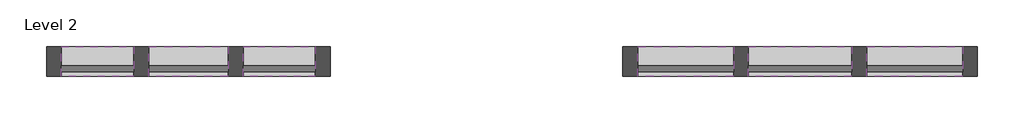
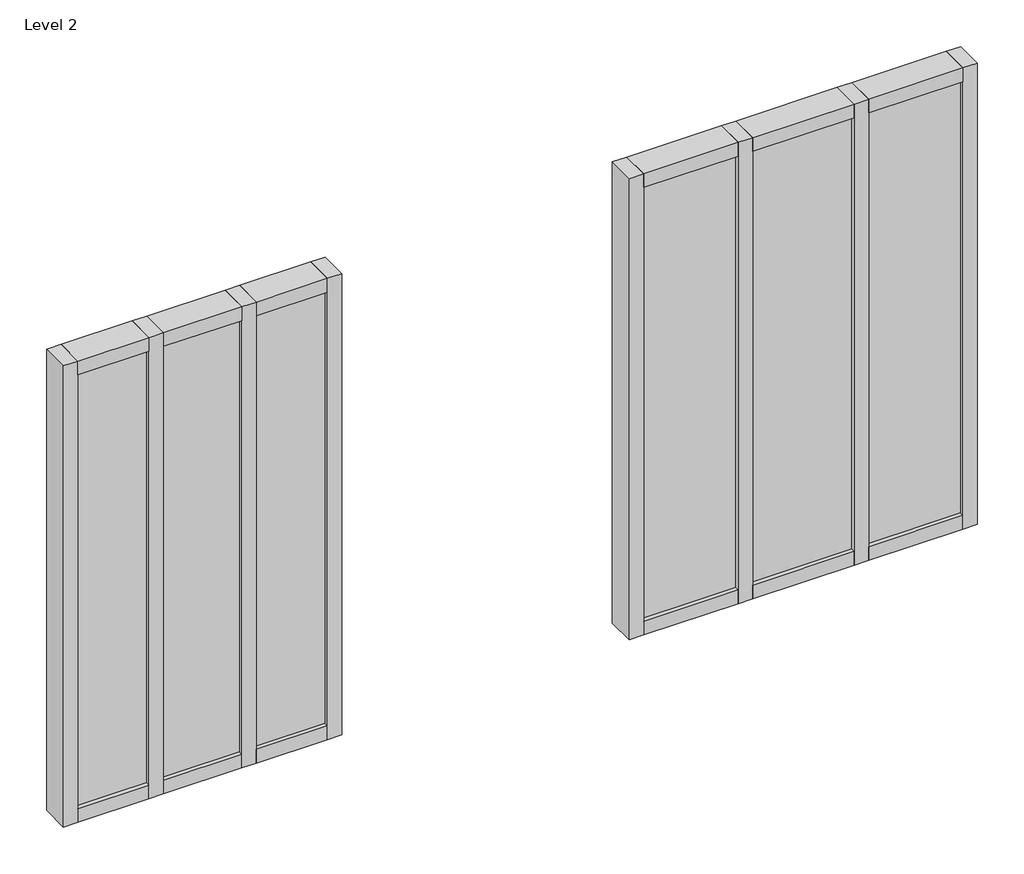
# One storey: 20 members, 6 plates.
"""IFC4 building model written with IfcOpenShell, lengths in millimetres."""

from ifc_helpers import new_model, si_unit, origin, place, context, project, spatial, transform, mapped, element, save
from components import member_dc106669, member_bc7dbe04, member_7cbddb58, member_3374d9b6, member_5ad95953, member_ff1b7d8f, system_panel_glazed_74c9e8f4, system_panel_glazed_660eca69, system_panel_glazed_45f6ab2d, system_panel_glazed_d43c1d57

model = new_model("IFC4")

# Units and contexts
model_context = context("Model", 3, world=origin())
ifc_project = project(units=[si_unit("LENGTHUNIT", "METRE", prefix="MILLI")], contexts=[model_context])

# Site, building, storey
site = spatial("IfcSite", under=ifc_project)
building = spatial("IfcBuilding", under=site)
storey = spatial("IfcBuildingStorey", under=building, Name="Level 2", Elevation=609.6)

# Members
placement = place(None, origin())
member_shape = member_dc106669(model_context)
element("IfcMember", 1, ObjectType="Rectangular Mullion : 2.5\" x 5\" rectangular", at=placement, inside=storey, context=model_context, shape_type="MappedRepresentation", body=[
    mapped(member_shape, transform((-8008.9218714, -2282.1569638, 2743.2), x_axis=(0.0, 0.0, 1.0), y_axis=(0.0, 1.0, 0.0), z_axis=(-1.0, 0.0, 0.0))),
])
element("IfcMember", 2, ObjectType="Rectangular Mullion : 2.5\" x 5\" rectangular", at=placement, inside=storey, context=model_context, shape_type="MappedRepresentation", body=[
    mapped(member_shape, transform((-7024.6718714, -2282.1569638, 2743.2), x_axis=(0.0, 0.0, 1.0), y_axis=(0.0, 1.0, 0.0), z_axis=(-1.0, 0.0, 0.0))),
])
element("IfcMember", 3, ObjectType="Rectangular Mullion : 2.5\" x 5\" rectangular", at=placement, inside=storey, context=model_context, shape_type="MappedRepresentation", body=[
    mapped(member_shape, transform((-6611.9218714, -2282.1569638, 609.6), x_axis=(0.0, 0.0, -1.0), y_axis=(0.0, 1.0, 0.0), z_axis=(1.0, 0.0, 0.0))),
])
element("IfcMember", 4, ObjectType="Rectangular Mullion : 2.5\" x 5\" rectangular", at=placement, inside=storey, context=model_context, shape_type="MappedRepresentation", body=[
    mapped(member_shape, transform((-7596.1718714, -2282.1569638, 609.6), x_axis=(0.0, 0.0, -1.0), y_axis=(0.0, 1.0, 0.0), z_axis=(1.0, 0.0, 0.0))),
])
member_2_shape = member_bc7dbe04(model_context)
element("IfcMember", 5, ObjectType="Rectangular Mullion : 2.5\" x 5\" rectangular", at=placement, inside=storey, context=model_context, shape_type="MappedRepresentation", body=[
    mapped(member_2_shape, transform((-7088.1718714, -2282.1569638, 609.6), x_axis=(0.0, 0.0, -1.0), y_axis=(0.0, 1.0, 0.0), z_axis=(1.0, 0.0, 0.0))),
])
element("IfcMember", 6, ObjectType="Rectangular Mullion : 2.5\" x 5\" rectangular", at=placement, inside=storey, context=model_context, shape_type="MappedRepresentation", body=[
    mapped(member_2_shape, transform((-7532.6718714, -2282.1569638, 2743.2), x_axis=(0.0, 0.0, 1.0), y_axis=(0.0, 1.0, 0.0), z_axis=(-1.0, 0.0, 0.0))),
])
member_3_shape = member_7cbddb58(model_context)
element("IfcMember", 7, ObjectType="Rectangular Mullion : 2.5\" x 5\" rectangular", at=placement, inside=storey, context=model_context, shape_type="MappedRepresentation", body=[
    mapped(member_3_shape, transform((-7564.4218714, -2282.1569638, 609.6), x_axis=(-1.0, 0.0, 0.0), y_axis=(0.0, 1.0, 0.0), z_axis=(0.0, 0.0, -1.0))),
])
element("IfcMember", 8, ObjectType="Rectangular Mullion : 2.5\" x 5\" rectangular", at=placement, inside=storey, context=model_context, shape_type="MappedRepresentation", body=[
    mapped(member_3_shape, transform((-7056.4218714, -2282.1569638, 609.6), x_axis=(-1.0, 0.0, 0.0), y_axis=(0.0, 1.0, 0.0), z_axis=(0.0, 0.0, -1.0))),
])
element("IfcMember", 9, ObjectType="Rectangular Mullion : 2.5\" x 5\" rectangular", at=placement, inside=storey, context=model_context, shape_type="MappedRepresentation", body=[
    mapped(member_3_shape, transform((-10142.5218714, -2282.1569638, 609.6), x_axis=(-1.0, 0.0, 0.0), y_axis=(0.0, 1.0, 0.0), z_axis=(0.0, 0.0, -1.0))),
])
element("IfcMember", 10, ObjectType="Rectangular Mullion : 2.5\" x 5\" rectangular", at=placement, inside=storey, context=model_context, shape_type="MappedRepresentation", body=[
    mapped(member_3_shape, transform((-9736.1218714, -2282.1569638, 609.6), x_axis=(-1.0, 0.0, 0.0), y_axis=(0.0, 1.0, 0.0), z_axis=(0.0, 0.0, -1.0))),
])
member_4_shape = member_3374d9b6(model_context)
element("IfcMember", 11, ObjectType="Rectangular Mullion : 2.5\" x 5\" rectangular", at=placement, inside=storey, context=model_context, shape_type="MappedRepresentation", body=[
    mapped(member_4_shape, transform((-6548.4218714, -2282.1569638, 2743.2), x_axis=(1.0, 0.0, 0.0), y_axis=(0.0, 1.0, 0.0), z_axis=(0.0, 0.0, 1.0))),
])
element("IfcMember", 12, ObjectType="Rectangular Mullion : 2.5\" x 5\" rectangular", at=placement, inside=storey, context=model_context, shape_type="MappedRepresentation", body=[
    mapped(member_4_shape, transform((-9329.7218714, -2282.1569638, 2743.2), x_axis=(1.0, 0.0, 0.0), y_axis=(0.0, 1.0, 0.0), z_axis=(0.0, 0.0, 1.0))),
])
element("IfcMember", 13, ObjectType="Rectangular Mullion : 2.5\" x 5\" rectangular", at=placement, inside=storey, context=model_context, shape_type="MappedRepresentation", body=[
    mapped(member_4_shape, transform((-8072.4218714, -2282.1569638, 609.6), x_axis=(-1.0, 0.0, 0.0), y_axis=(0.0, 1.0, 0.0), z_axis=(0.0, 0.0, -1.0))),
])
element("IfcMember", 14, ObjectType="Rectangular Mullion : 2.5\" x 5\" rectangular", at=placement, inside=storey, context=model_context, shape_type="MappedRepresentation", body=[
    mapped(member_4_shape, transform((-10548.9218714, -2282.1569638, 609.6), x_axis=(-1.0, 0.0, 0.0), y_axis=(0.0, 1.0, 0.0), z_axis=(0.0, 0.0, -1.0))),
])
member_5_shape = member_5ad95953(model_context)
element("IfcMember", 15, ObjectType="Rectangular Mullion : 2.5\" x 5\" rectangular", at=placement, inside=storey, context=model_context, shape_type="MappedRepresentation", body=[
    mapped(member_5_shape, transform((-10485.4218714, -2282.1569638, 2743.2), x_axis=(0.0, 0.0, 1.0), y_axis=(0.0, 1.0, 0.0), z_axis=(-1.0, 0.0, 0.0))),
])
element("IfcMember", 16, ObjectType="Rectangular Mullion : 2.5\" x 5\" rectangular", at=placement, inside=storey, context=model_context, shape_type="MappedRepresentation", body=[
    mapped(member_5_shape, transform((-9704.3718714, -2282.1569638, 2743.2), x_axis=(0.0, 0.0, 1.0), y_axis=(0.0, 1.0, 0.0), z_axis=(-1.0, 0.0, 0.0))),
])
element("IfcMember", 17, ObjectType="Rectangular Mullion : 2.5\" x 5\" rectangular", at=placement, inside=storey, context=model_context, shape_type="MappedRepresentation", body=[
    mapped(member_5_shape, transform((-9393.2218714, -2282.1569638, 609.6), x_axis=(0.0, 0.0, -1.0), y_axis=(0.0, 1.0, 0.0), z_axis=(1.0, 0.0, 0.0))),
])
element("IfcMember", 18, ObjectType="Rectangular Mullion : 2.5\" x 5\" rectangular", at=placement, inside=storey, context=model_context, shape_type="MappedRepresentation", body=[
    mapped(member_5_shape, transform((-10174.2718714, -2282.1569638, 609.6), x_axis=(0.0, 0.0, -1.0), y_axis=(0.0, 1.0, 0.0), z_axis=(1.0, 0.0, 0.0))),
])
member_6_shape = member_ff1b7d8f(model_context)
element("IfcMember", 19, ObjectType="Rectangular Mullion : 2.5\" x 5\" rectangular", at=placement, inside=storey, context=model_context, shape_type="MappedRepresentation", body=[
    mapped(member_6_shape, transform((-9767.8718714, -2282.1569638, 609.6), x_axis=(0.0, 0.0, -1.0), y_axis=(0.0, 1.0, 0.0), z_axis=(1.0, 0.0, 0.0))),
])
element("IfcMember", 20, ObjectType="Rectangular Mullion : 2.5\" x 5\" rectangular", at=placement, inside=storey, context=model_context, shape_type="MappedRepresentation", body=[
    mapped(member_6_shape, transform((-10110.7718714, -2282.1569638, 2743.2), x_axis=(0.0, 0.0, 1.0), y_axis=(0.0, 1.0, 0.0), z_axis=(-1.0, 0.0, 0.0))),
])

# Plates
system_panel_glazed_shape = system_panel_glazed_74c9e8f4(model_context)
element("IfcPlate", 21, ObjectType="System Panel : Glazed", at=placement, inside=storey, context=model_context, shape_type="MappedRepresentation", body=[
    mapped(system_panel_glazed_shape, transform((-6818.2968714, -2282.1569638, 673.1), x_axis=(-1.0, 0.0, 0.0), y_axis=(0.0, -1.0, 0.0), z_axis=(0.0, 0.0, 1.0))),
])
element("IfcPlate", 22, ObjectType="System Panel : Glazed", at=placement, inside=storey, context=model_context, shape_type="MappedRepresentation", body=[
    mapped(system_panel_glazed_shape, transform((-7802.5468714, -2282.1569638, 673.1), x_axis=(-1.0, 0.0, 0.0), y_axis=(0.0, -1.0, 0.0), z_axis=(0.0, 0.0, 1.0))),
])
system_panel_glazed_2_shape = system_panel_glazed_660eca69(model_context)
element("IfcPlate", 23, ObjectType="System Panel : Glazed", at=placement, inside=storey, context=model_context, shape_type="MappedRepresentation", body=[
    mapped(system_panel_glazed_2_shape, transform((-7310.4218714, -2282.1569638, 673.1), x_axis=(-1.0, 0.0, 0.0), y_axis=(0.0, -1.0, 0.0), z_axis=(0.0, 0.0, 1.0))),
])
system_panel_glazed_3_shape = system_panel_glazed_45f6ab2d(model_context)
element("IfcPlate", 24, ObjectType="System Panel : Glazed", at=placement, inside=storey, context=model_context, shape_type="MappedRepresentation", body=[
    mapped(system_panel_glazed_3_shape, transform((-9548.7968714, -2282.1569638, 673.1), x_axis=(-1.0, 0.0, 0.0), y_axis=(0.0, -1.0, 0.0), z_axis=(0.0, 0.0, 1.0))),
])
element("IfcPlate", 25, ObjectType="System Panel : Glazed", at=placement, inside=storey, context=model_context, shape_type="MappedRepresentation", body=[
    mapped(system_panel_glazed_3_shape, transform((-10329.8468714, -2282.1569638, 673.1), x_axis=(-1.0, 0.0, 0.0), y_axis=(0.0, -1.0, 0.0), z_axis=(0.0, 0.0, 1.0))),
])
system_panel_glazed_4_shape = system_panel_glazed_d43c1d57(model_context)
element("IfcPlate", 26, ObjectType="System Panel : Glazed", at=placement, inside=storey, context=model_context, shape_type="MappedRepresentation", body=[
    mapped(system_panel_glazed_4_shape, transform((-9939.3218714, -2282.1569638, 673.1), x_axis=(-1.0, 0.0, 0.0), y_axis=(0.0, -1.0, 0.0), z_axis=(0.0, 0.0, 1.0))),
])

save(model, "model.ifc")

# Revit data of these elements
# Type "Rectangular Mullion : 2.5\" x 5\" rectangular"
#   built-in parameter 1007304 = 0.416667 (stored number, unit not read)
#   built-in parameter 1007301 = 0.104167 (stored number, unit not read)
#   built-in parameter 1007300 = 0.104167 (stored number, unit not read)
# Type "System Panel : Glazed"
#   Construction Type Id = "GSP4R"
#   Analytic Construction = "1/8 in Pilkington single glazing"
#   Visual Light Transmittance = 0.9
#   Solar Heat Gain Coefficient = 0.86
#   Heat Transfer Coefficient (U) = 1.18115 BTU/(h·ft²·°F)
#   Define Thermal Properties by = 1
# Elements 1, 2, 3, 4, 5, 6, 7, 8, 9, 10, 11, 12, 13, 14, 15, 16, 17, 18, 19, 20 (IfcMember, "Rectangular Mullion : 2.5\" x 5\" rectangular")
#   Phase Created = New Construction
# Elements 21, 22, 23, 24, 25, 26 (IfcPlate, "System Panel : Glazed")
#   Phase Created = New Construction
#   Materials on its faces: "Glass"
# Materials
#   "Glass": class "Glass", colour RGB 0 128 192, transparency 0.75, Description = "Soda Lime Glass", Cost = 0
